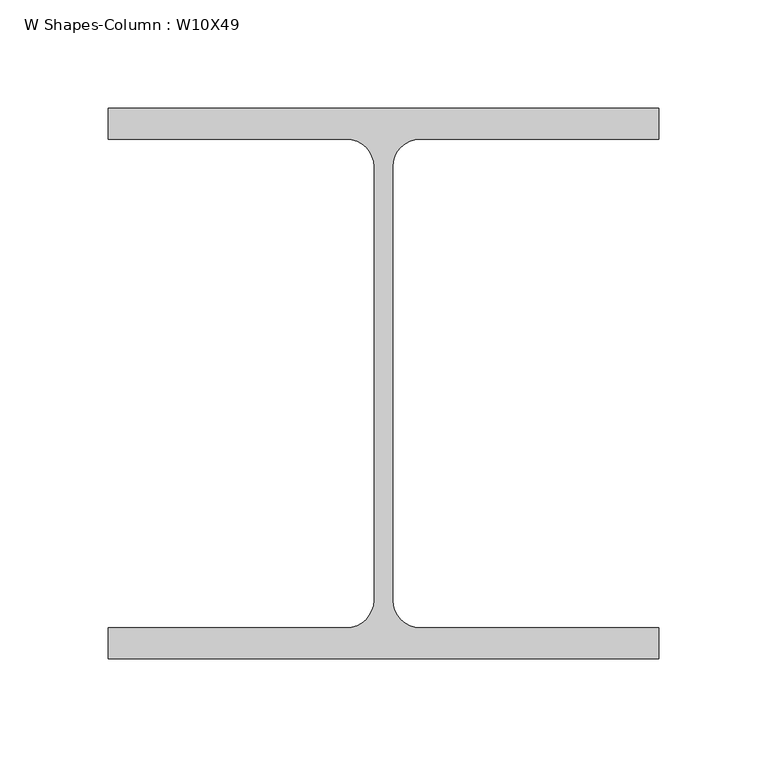
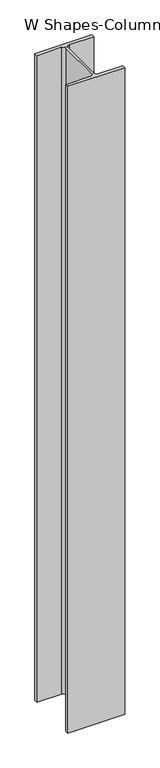
"""IFC4 building model written with IfcOpenShell, lengths in millimetres: column geometry, W Shapes-Column : W10X49."""

from ifc_helpers import new_model, si_unit, point, frame, frame_2d, origin, place, context, project, spatial, polyline, circle_curve, trimmed, segment, composite_curve, outline, extrude, source, transform, mapped, element, save


def w_shapes_column_w10x49_ceff5d29(model_context):
    return source(origin(), model_context, "Body", "SweptSolid", [
        extrude(outline(composite_curve([segment(polyline([(127.0, 127.0), (127.0, 112.776), (17.018, 112.776)]), True, "CONTINUOUS"), segment(trimmed(circle_curve(frame_2d((17.018, 100.076)), 12.7), [point((17.018, 112.776))], [point((4.318, 100.076))], True, "CARTESIAN"), True, "CONTINUOUS"), segment(polyline([(4.318, 100.076), (4.318, -100.076)]), True, "CONTINUOUS"), segment(trimmed(circle_curve(frame_2d((17.018, -100.076)), 12.7), [point((4.318, -100.076))], [point((17.018, -112.776))], True, "CARTESIAN"), True, "CONTINUOUS"), segment(polyline([(17.018, -112.776), (127.0, -112.776), (127.0, -127.0), (-127.0, -127.0), (-127.0, -112.776), (-17.018, -112.776)]), True, "CONTINUOUS"), segment(trimmed(circle_curve(frame_2d((-17.018, -100.076)), 12.7), [point((-17.018, -112.776))], [point((-4.318, -100.076))], True, "CARTESIAN"), True, "CONTINUOUS"), segment(polyline([(-4.318, -100.076), (-4.318, 100.076)]), True, "CONTINUOUS"), segment(trimmed(circle_curve(frame_2d((-17.018, 100.076)), 12.7), [point((-4.318, 100.076))], [point((-17.018, 112.776))], True, "CARTESIAN"), True, "CONTINUOUS"), segment(polyline([(-17.018, 112.776), (-127.0, 112.776), (-127.0, 127.0), (127.0, 127.0)]), True, "CONTINUOUS")], self_intersect=False)), frame((0.0, 0.0, 3048.0), z_axis=(0.0, 0.0, 1.0), x_axis=(1.0, 0.0, 0.0)), (0.0, 0.0, 1.0), 3048.0),
    ])


if __name__ == "__main__":
    model = new_model("IFC4")
    model_context = context("Model", 3, world=origin())
    ifc_project = project(units=[si_unit("LENGTHUNIT", "METRE", prefix="MILLI")], contexts=[model_context])
    site = spatial("IfcSite", under=ifc_project)
    building = spatial("IfcBuilding", under=site)
    placement = place(None, origin())
    w_shapes_column_w10x49_shape = w_shapes_column_w10x49_ceff5d29(model_context)
    element("IfcColumn", 1, ObjectType="W Shapes-Column : W10X49", at=placement, inside=building, context=model_context, shape_type="MappedRepresentation", body=[
        mapped(w_shapes_column_w10x49_shape, transform((0.0, 0.0, 0.0), x_axis=(1.0, 0.0, 0.0), y_axis=(0.0, 1.0, 0.0), z_axis=(0.0, 0.0, 1.0))),
    ])
    save(model, "model.ifc")

# Revit data of these elements
# Type "W Shapes-Column : W10X49"
#   Section Name Key = "W10x49"
#   Assembly Code = "B10"
#   Width = 10.000"
#   Web Thickness = 0.340"
#   Web Fillet = 0.500"
#   Warping Constant = 2070.00 in⁶
#   Torsional Moment of Inertia = 1.39 in⁴
#   Section Area = 14.40 in²
#   Plastic Modulus weak axis = 28.30 in³
#   Plastic Modulus strong axis = 60.40 in³
#   Perimeter = 58.50 ft²/ft
#   Nominal Weight = 49.00 lbf/ft
#   Moment of Inertia weak axis = 93.40 in⁴
#   Moment of Inertia strong axis = 272.00 in⁴
#   Height = 10.000"
#   Flange Thickness = 0.560"
#   Elastic Modulus weak axis = 18.70 in³
#   Elastic Modulus strong axis = 54.60 in³
#   Centroid Vertical = 5.000"
#   Centroid Horizontal = 5.000"
#   Structural Material [instance default] = Steel ASTM A992
#   Principal Axes Angle = 0
# Element 1 (IfcColumn, "W Shapes-Column : W10X49")
#   Materials on its faces: "Steel ASTM A992"
# Materials
#   "Steel ASTM A992": class "Metal", colour RGB 199 199 199, transparency 0, Description = "Structural steel 50ksi", Cost = 0
